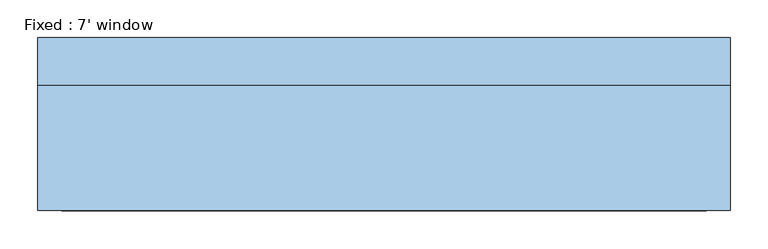
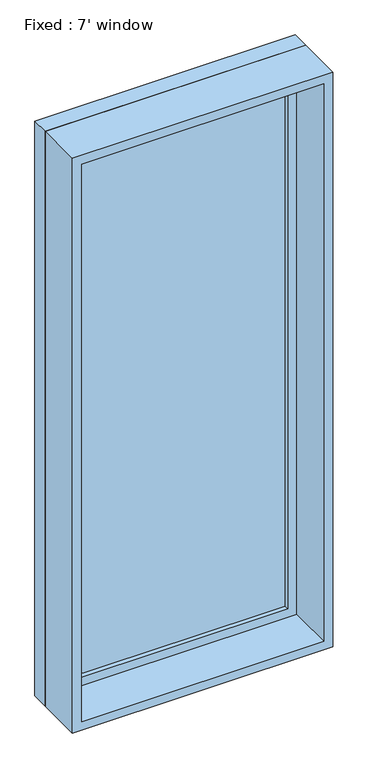
"""IFC4 building model written with IfcOpenShell, lengths in millimetres: window geometry, Fixed : 7' window."""

from ifc_helpers import new_model, si_unit, frame, origin, place, context, project, spatial, polyline, outline, extrude, source, transform, mapped, element, save


def fixed_7_window_d95a62fe(model_context):
    return source(origin(), model_context, "Body", "SweptSolid", [
        extrude(outline(polyline([(355.6, 66.675), (-431.8, 66.675), (-431.8, 79.375), (355.6, 79.375), (355.6, 66.675)])), frame((0.0, 0.0, 977.9), z_axis=(0.0, 0.0, 1.0), x_axis=(1.0, 0.0, 0.0)), (0.0, 0.0, 1.0), 2006.6),
        extrude(outline(polyline([(3028.95, -476.25), (933.45, -476.25), (933.45, 400.05), (3028.95, 400.05), (3028.95, -476.25)]), holes=[polyline([(2984.5, -431.8), (2984.5, 355.6), (977.9, 355.6), (977.9, -431.8), (2984.5, -431.8)])]), frame((0.0, 50.8, 0.0), z_axis=(0.0, 1.0, 0.0), x_axis=(0.0, 0.0, 1.0)), (0.0, 0.0, 1.0), 44.45),
        extrude(outline(polyline([(3048.0, -495.3), (914.4, -495.3), (914.4, 419.1), (3048.0, 419.1), (3048.0, -495.3)]), holes=[polyline([(3016.25, -463.55), (3016.25, 387.35), (946.15, 387.35), (946.15, -463.55), (3016.25, -463.55)])]), frame((0.0, -114.3, 0.0), z_axis=(0.0, 1.0, 0.0), x_axis=(0.0, 0.0, 1.0)), (0.0, 0.0, 1.0), 165.1),
        extrude(outline(polyline([(3048.0, 419.1), (3048.0, -495.3), (914.4, -495.3), (914.4, 419.1), (3048.0, 419.1)]), holes=[polyline([(3028.95, 400.05), (933.45, 400.05), (933.45, -476.25), (3028.95, -476.25), (3028.95, 400.05)])]), frame((0.0, 50.8, 0.0), z_axis=(0.0, 1.0, 0.0), x_axis=(0.0, 0.0, 1.0)), (0.0, 0.0, 1.0), 63.5),
    ])


if __name__ == "__main__":
    model = new_model("IFC4")
    model_context = context("Model", 3, world=origin())
    ifc_project = project(units=[si_unit("LENGTHUNIT", "METRE", prefix="MILLI")], contexts=[model_context])
    site = spatial("IfcSite", under=ifc_project)
    building = spatial("IfcBuilding", under=site)
    placement = place(None, origin())
    fixed_7_window_shape = fixed_7_window_d95a62fe(model_context)
    element("IfcWindow", 1, ObjectType="Fixed : 7' window", at=placement, inside=building, context=model_context, shape_type="MappedRepresentation", body=[
        mapped(fixed_7_window_shape, transform((0.0, 0.0, 0.0), x_axis=(1.0, 0.0, 0.0), y_axis=(0.0, 1.0, 0.0), z_axis=(0.0, 0.0, 1.0))),
    ])
    save(model, "model.ifc")

# Revit data of these elements
# Type "Fixed : 7' window"
#   Type Mark = "18"
#   Construction Type Id = "GSP4R"
#   Assembly Code = "B2020100"
#   Analytic Construction = "1/8 in Pilkington single glazing"
#   Visual Light Transmittance = 0.9
#   Solar Heat Gain Coefficient = 0.78
#   Heat Transfer Coefficient (U) = 0.6496 BTU/(h·ft²·°F)
#   Height = 7' - 0"
#   Default Sill Height = 3' - 0"
#   Width = 3' - 0"
#   Window Inset = 0' - 0 3/4"
#   Define Thermal Properties by = 1
#   Glass Pane Material = Glass
#   Sash Material = Sash
#   Wall Closure = (empty or 0)
# Element 1 (IfcWindow, "Fixed : 7' window")
#   Materials on its faces: "Sash", "Glass"
# Materials
#   "Glass": class "Glass", colour RGB 0 128 192, transparency 0.75, Description = "Soda Lime Glass", Cost = 0
#   "Sash": class "Wood", colour RGB 224 178 126, transparency 0, Cost = 0
